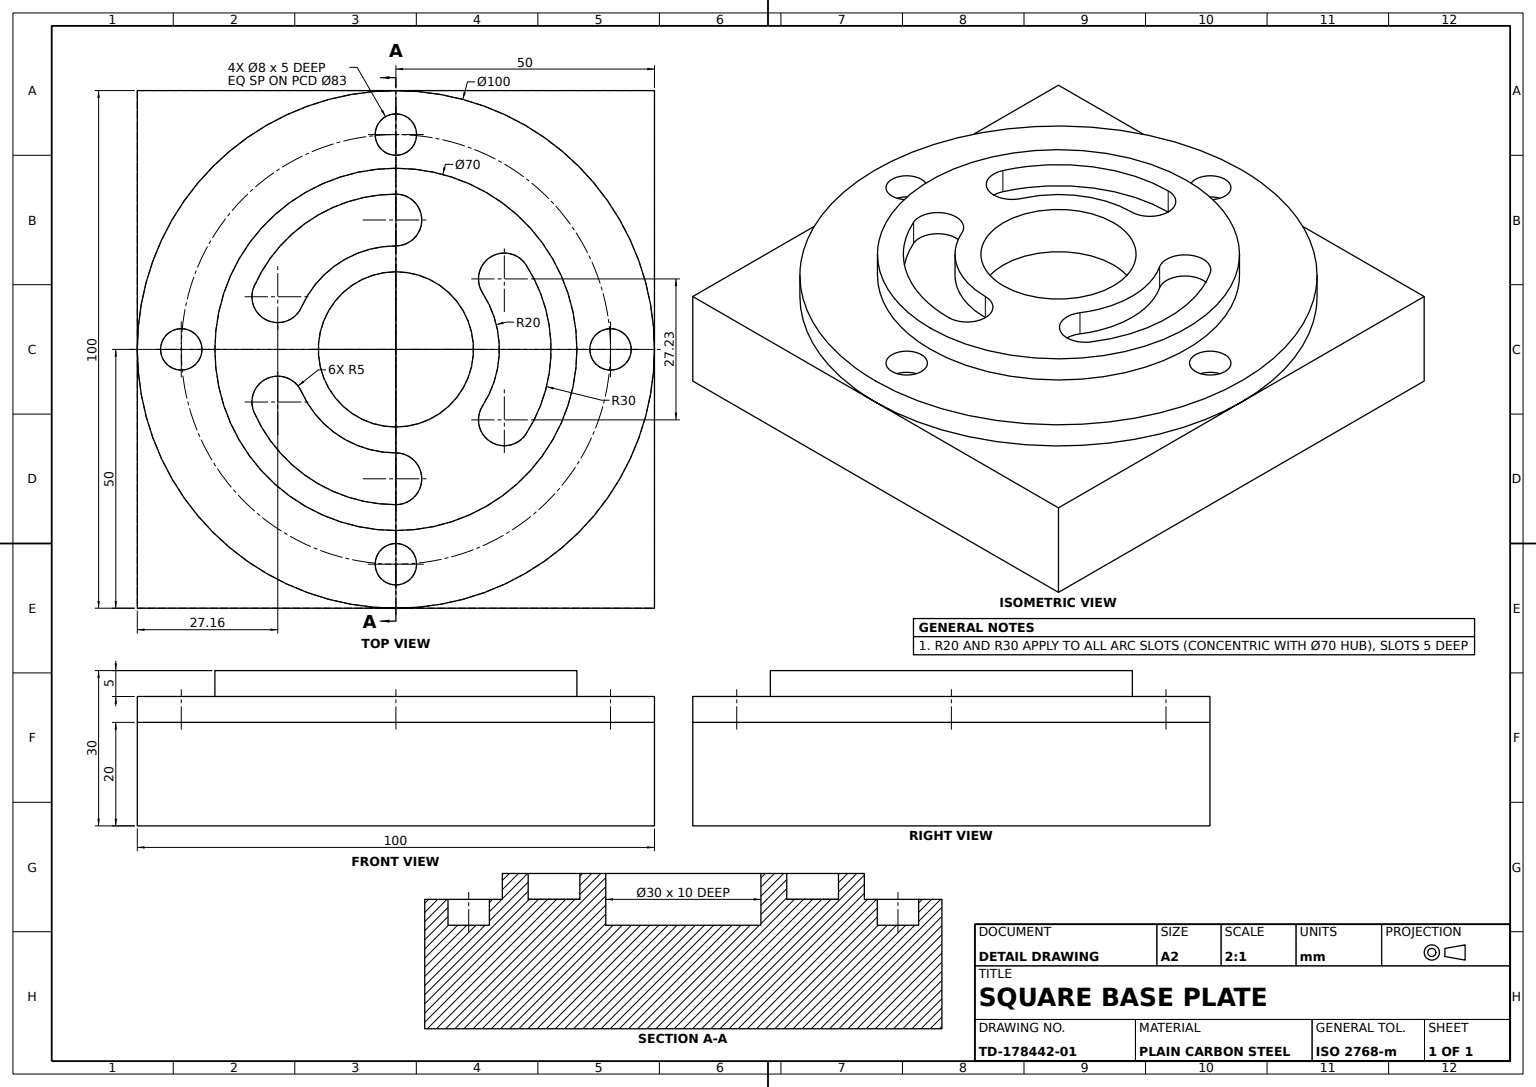
from build123d import *

# Parameters (mm, degrees)
BASE_PLATE_SKETCH_W     = 100
BASE_PLATE_SKETCH_H     = 100
BASE_PLATE_DEPTH        = 20
FLANGE_DISC_SKETCH_R    = 50
FLANGE_DISC_DEPTH       = 5
FLANGE_HOLES_SKETCH_R   = 4
FLANGE_HOLES_4X_8_DEPTH = 5
HUB_DISC_SKETCH_R       = 35
HUB_DISC_DEPTH          = 5
ARC_SLOTS_3X_DEPTH      = 5
CENTRE_BORE_SKETCH_R    = 15
CENTRE_BORE_DEPTH       = 10


with BuildPart() as part:
    # Base Plate Sketch → Base Plate (new body)
    with BuildSketch(Plane(origin=(0, 0, 0), x_dir=(1, 0, 0), z_dir=(0, 1, 0))):
        Rectangle(BASE_PLATE_SKETCH_W, BASE_PLATE_SKETCH_H)
    extrude(amount=BASE_PLATE_DEPTH)

    # Flange Disc Sketch → Flange Disc (add)
    with BuildSketch(Plane(origin=(0, 20, 0), x_dir=(1, 0, 0), z_dir=(0, 1, 0))):
        with Locations(Location((0, 0, 0), (0, 0, 270))):
            Circle(FLANGE_DISC_SKETCH_R)
    extrude(amount=FLANGE_DISC_DEPTH)

    # Flange Holes Sketch → Flange Holes 4xØ8 (cut)
    with BuildSketch(Plane(origin=(0, 25, 0), x_dir=(1, 0, 0), z_dir=(0, 1, 0))):
        with Locations(Location((0, 41.5, 0), (0, 0, 270))):
            Circle(FLANGE_HOLES_SKETCH_R)
        with Locations(Location((41.5, 0, 0), (0, 0, 270))):
            Circle(FLANGE_HOLES_SKETCH_R)
        with Locations(Location((0, -41.5, 0), (0, 0, 270))):
            Circle(FLANGE_HOLES_SKETCH_R)
        with Locations(Location((-41.5, 0, 0), (0, 0, 270))):
            Circle(FLANGE_HOLES_SKETCH_R)
    extrude(amount=-FLANGE_HOLES_4X_8_DEPTH, mode=Mode.SUBTRACT)

    # Hub Disc Sketch → Hub Disc (add)
    with BuildSketch(Plane(origin=(0, 25, 0), x_dir=(1, 0, 0), z_dir=(0, 1, 0))):
        with Locations(Location((0, 0, 0), (0, 0, 270))):
            Circle(HUB_DISC_SKETCH_R)
    extrude(amount=HUB_DISC_DEPTH)

    # Arc Slots Sketch → Arc Slots 3x (cut)
    with BuildSketch(Plane(origin=(0, 30, 0), x_dir=(1, 0, 0), z_dir=(0, 1, 0))):
        with BuildLine():
            ThreePointArc((-27.405227761, -12.2046504), (-16.338, -25.160877489), (0, -30))
            ThreePointArc((0, -30), (5, -25), (0, -20))
            ThreePointArc((0, -20), (-10.892, -16.773918326), (-18.27015184, -8.1364336))
            ThreePointArc((-18.27015184, -8.1364336), (-24.871798201, -5.60300404), (-27.405227761, -12.2046504))
        make_face()
        with BuildLine():
            ThreePointArc((16.773411359, 10.8927807), (18.243569024, 17.809328715), (25.160117038, 16.33917105))
            ThreePointArc((25.160117038, 16.33917105), (30, 0), (25.160117038, -16.33917105))
            ThreePointArc((25.160117038, -16.33917105), (18.243569024, -17.809328715), (16.773411359, -10.8927807))
            ThreePointArc((16.773411359, -10.8927807), (20, 0), (16.773411359, 10.8927807))
        make_face()
        with BuildLine():
            ThreePointArc((0, 30), (5, 25), (0, 20))
            ThreePointArc((0, 20), (-10.892, 16.773918326), (-18.27015184, 8.1364336))
            ThreePointArc((-18.27015184, 8.1364336), (-24.871798201, 5.60300404), (-27.405227761, 12.2046504))
            ThreePointArc((-27.405227761, 12.2046504), (-16.338, 25.160877489), (0, 30))
        make_face()
    extrude(amount=-ARC_SLOTS_3X_DEPTH, mode=Mode.SUBTRACT)

    # Centre Bore Sketch → Centre Bore (cut)
    with BuildSketch(Plane(origin=(0, 30, 0), x_dir=(1, 0, 0), z_dir=(0, 1, 0))):
        with Locations(Location((0, 0, 0), (0, 0, 270))):
            Circle(CENTRE_BORE_SKETCH_R)
    extrude(amount=-CENTRE_BORE_DEPTH, mode=Mode.SUBTRACT)


solid = part.part
